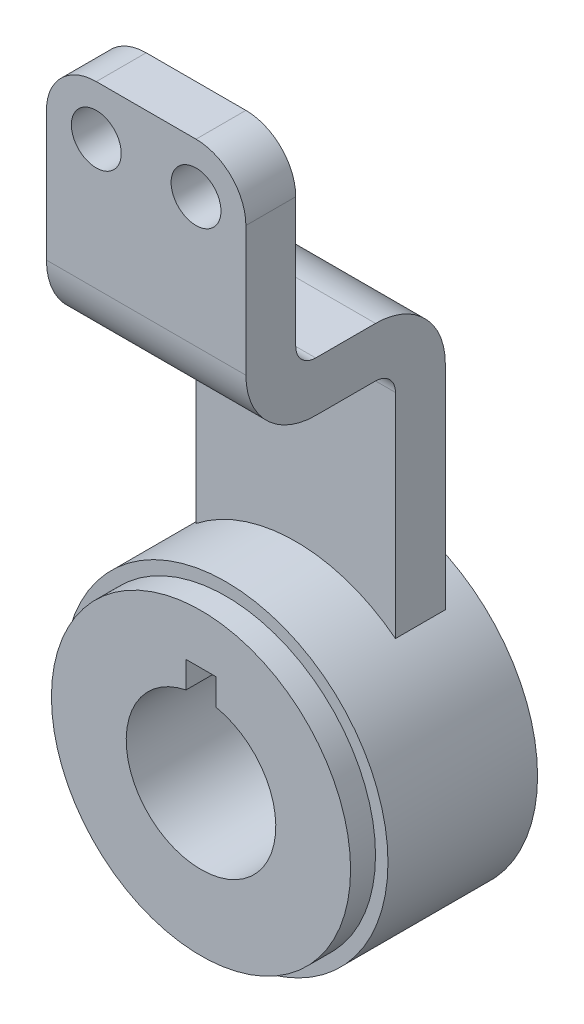
ISO-10303-21;
HEADER;
FILE_DESCRIPTION(('STEP AP214'),'2;1');
FILE_NAME('part.step','',(''),(''),'','','');
FILE_SCHEMA(('AUTOMOTIVE_DESIGN { 1 0 10303 214 1 1 1 1 }'));
ENDSEC;
DATA;
#1=APPLICATION_CONTEXT('core data for automotive mechanical design processes');
#2=APPLICATION_PROTOCOL_DEFINITION('international standard','automotive_design',2000,#1);
#3=PRODUCT_CONTEXT('',#1,'mechanical');
#4=PRODUCT('Part','Part','',(#3));
#5=PRODUCT_RELATED_PRODUCT_CATEGORY('part','',(#4));
#6=PRODUCT_DEFINITION_FORMATION('','',#4);
#7=PRODUCT_DEFINITION_CONTEXT('part definition',#1,'design');
#8=PRODUCT_DEFINITION('design','',#6,#7);
#9=PRODUCT_DEFINITION_SHAPE('','',#8);
#10=(LENGTH_UNIT() NAMED_UNIT(*) SI_UNIT(.MILLI.,.METRE.));
#11=(NAMED_UNIT(*) PLANE_ANGLE_UNIT() SI_UNIT($,.RADIAN.));
#12=(NAMED_UNIT(*) SI_UNIT($,.STERADIAN.) SOLID_ANGLE_UNIT());
#13=UNCERTAINTY_MEASURE_WITH_UNIT(LENGTH_MEASURE(1.E-05),#10,'distance_accuracy_value','');
#14=(GEOMETRIC_REPRESENTATION_CONTEXT(3) GLOBAL_UNCERTAINTY_ASSIGNED_CONTEXT((#13)) GLOBAL_UNIT_ASSIGNED_CONTEXT((#10,
#11,#12)) REPRESENTATION_CONTEXT('',''));
#15=CARTESIAN_POINT('',(0.,0.,0.));
#16=DIRECTION('',(0.,0.,1.));
#17=DIRECTION('',(1.,0.,0.));
#18=AXIS2_PLACEMENT_3D('',#15,#16,#17);
#19=CARTESIAN_POINT('',(0.,0.,16.));
#20=DIRECTION('',(0.,0.,1.));
#21=DIRECTION('',(1.,0.,0.));
#22=AXIS2_PLACEMENT_3D('',#19,#20,#21);
#23=PLANE('',#22);
#24=DIRECTION('',(0.,1.,0.));
#25=VECTOR('',#24,1.);
#26=CARTESIAN_POINT('',(20.,82.3606797749979,16.));
#27=LINE('',#26,#25);
#28=CARTESIAN_POINT('',(20.,25.617376914899,16.));
#29=VERTEX_POINT('',#28);
#30=CARTESIAN_POINT('',(20.,68.3606797749979,16.));
#31=VERTEX_POINT('',#30);
#32=EDGE_CURVE('E172',#29,#31,#27,.T.);
#33=ORIENTED_EDGE('',*,*,#32,.T.);
#34=DIRECTION('',(-1.,0.,0.));
#35=VECTOR('',#34,1.);
#36=CARTESIAN_POINT('',(0.,68.3606797749979,16.));
#37=LINE('',#36,#35);
#38=CARTESIAN_POINT('',(-20.,68.3606797749979,16.));
#39=VERTEX_POINT('',#38);
#40=EDGE_CURVE('E241',#31,#39,#37,.T.);
#41=ORIENTED_EDGE('',*,*,#40,.T.);
#42=DIRECTION('',(0.,-1.,0.));
#43=VECTOR('',#42,1.);
#44=CARTESIAN_POINT('',(-20.,22.3606797749979,16.));
#45=LINE('',#44,#43);
#46=CARTESIAN_POINT('',(-20.,25.617376914899,16.));
#47=VERTEX_POINT('',#46);
#48=EDGE_CURVE('E286',#39,#47,#45,.T.);
#49=ORIENTED_EDGE('',*,*,#48,.T.);
#50=CARTESIAN_POINT('',(0.,0.,16.));
#51=DIRECTION('',(0.,0.,1.));
#52=DIRECTION('',(1.,0.,0.));
#53=AXIS2_PLACEMENT_3D('',#50,#51,#52);
#54=CIRCLE('',#53,32.5);
#55=EDGE_CURVE('E183',#29,#47,#54,.T.);
#56=ORIENTED_EDGE('',*,*,#55,.F.);
#57=EDGE_LOOP('',(#33,#41,#49,#56));
#58=FACE_BOUND('',#57,.T.);
#59=ADVANCED_FACE('F39',(#58),#23,.T.);
#60=CARTESIAN_POINT('',(0.,0.,30.));
#61=DIRECTION('',(0.,0.,1.));
#62=DIRECTION('',(1.,0.,0.));
#63=AXIS2_PLACEMENT_3D('',#60,#61,#62);
#64=PLANE('',#63);
#65=CARTESIAN_POINT('',(0.,0.,30.));
#66=DIRECTION('',(0.,0.,1.));
#67=DIRECTION('',(1.,0.,0.));
#68=AXIS2_PLACEMENT_3D('',#65,#66,#67);
#69=CIRCLE('',#68,30.);
#70=CARTESIAN_POINT('',(30.,0.,30.));
#71=VERTEX_POINT('',#70);
#72=EDGE_CURVE('E188',#71,#71,#69,.T.);
#73=ORIENTED_EDGE('',*,*,#72,.F.);
#74=EDGE_LOOP('',(#73));
#75=FACE_BOUND('',#74,.T.);
#76=CARTESIAN_POINT('',(0.,0.,30.));
#77=DIRECTION('',(0.,0.,1.));
#78=DIRECTION('',(1.,0.,0.));
#79=AXIS2_PLACEMENT_3D('',#76,#77,#78);
#80=CIRCLE('',#79,32.5);
#81=CARTESIAN_POINT('',(32.5,0.,30.));
#82=VERTEX_POINT('',#81);
#83=EDGE_CURVE('E194',#82,#82,#80,.T.);
#84=ORIENTED_EDGE('',*,*,#83,.T.);
#85=EDGE_LOOP('',(#84));
#86=FACE_BOUND('',#85,.T.);
#87=ADVANCED_FACE('F345',(#75,#86),#64,.T.);
#88=CARTESIAN_POINT('',(0.,0.,0.));
#89=DIRECTION('',(0.,0.,1.));
#90=DIRECTION('',(1.,0.,0.));
#91=AXIS2_PLACEMENT_3D('',#88,#89,#90);
#92=PLANE('',#91);
#93=CARTESIAN_POINT('',(0.,0.,0.));
#94=DIRECTION('',(0.,0.,1.));
#95=DIRECTION('',(1.,0.,0.));
#96=AXIS2_PLACEMENT_3D('',#93,#94,#95);
#97=CIRCLE('',#96,32.5);
#98=CARTESIAN_POINT('',(32.5,0.,0.));
#99=VERTEX_POINT('',#98);
#100=EDGE_CURVE('E199',#99,#99,#97,.T.);
#101=ORIENTED_EDGE('',*,*,#100,.F.);
#102=EDGE_LOOP('',(#101));
#103=FACE_BOUND('',#102,.T.);
#104=DIRECTION('',(0.,1.,0.));
#105=VECTOR('',#104,1.);
#106=CARTESIAN_POINT('',(3.,14.6969384566991,0.));
#107=LINE('',#106,#105);
#108=CARTESIAN_POINT('',(3.,14.6969384566991,0.));
#109=VERTEX_POINT('',#108);
#110=CARTESIAN_POINT('',(3.,20.,0.));
#111=VERTEX_POINT('',#110);
#112=EDGE_CURVE('E309',#109,#111,#107,.T.);
#113=ORIENTED_EDGE('',*,*,#112,.T.);
#114=DIRECTION('',(-1.,0.,0.));
#115=VECTOR('',#114,1.);
#116=CARTESIAN_POINT('',(-3.,20.,0.));
#117=LINE('',#116,#115);
#118=CARTESIAN_POINT('',(-3.,20.,0.));
#119=VERTEX_POINT('',#118);
#120=EDGE_CURVE('E313',#111,#119,#117,.T.);
#121=ORIENTED_EDGE('',*,*,#120,.T.);
#122=DIRECTION('',(0.,-1.,0.));
#123=VECTOR('',#122,1.);
#124=CARTESIAN_POINT('',(-3.,14.6969384566991,0.));
#125=LINE('',#124,#123);
#126=CARTESIAN_POINT('',(-3.,14.6969384566991,0.));
#127=VERTEX_POINT('',#126);
#128=EDGE_CURVE('E320',#119,#127,#125,.T.);
#129=ORIENTED_EDGE('',*,*,#128,.T.);
#130=CARTESIAN_POINT('',(0.,0.,0.));
#131=DIRECTION('',(0.,0.,1.));
#132=DIRECTION('',(1.,0.,0.));
#133=AXIS2_PLACEMENT_3D('',#130,#131,#132);
#134=CIRCLE('',#133,15.);
#135=EDGE_CURVE('E318',#127,#109,#134,.T.);
#136=ORIENTED_EDGE('',*,*,#135,.T.);
#137=EDGE_LOOP('',(#113,#121,#129,#136));
#138=FACE_BOUND('',#137,.T.);
#139=ADVANCED_FACE('F339',(#103,#138),#92,.F.);
#140=CARTESIAN_POINT('',(0.,0.,30.));
#141=DIRECTION('',(0.,0.,-1.));
#142=DIRECTION('',(-1.,0.,0.));
#143=AXIS2_PLACEMENT_3D('',#140,#141,#142);
#144=CYLINDRICAL_SURFACE('',#143,32.5);
#145=DIRECTION('',(0.,0.,-1.));
#146=VECTOR('',#145,1.);
#147=CARTESIAN_POINT('',(20.,25.617376914899,30.));
#148=LINE('',#147,#146);
#149=CARTESIAN_POINT('',(20.,25.617376914899,6.));
#150=VERTEX_POINT('',#149);
#151=EDGE_CURVE('E184',#29,#150,#148,.T.);
#152=ORIENTED_EDGE('',*,*,#151,.F.);
#153=ORIENTED_EDGE('',*,*,#55,.T.);
#154=DIRECTION('',(0.,0.,-1.));
#155=VECTOR('',#154,1.);
#156=CARTESIAN_POINT('',(-20.,25.617376914899,30.));
#157=LINE('',#156,#155);
#158=CARTESIAN_POINT('',(-20.,25.617376914899,6.));
#159=VERTEX_POINT('',#158);
#160=EDGE_CURVE('E166',#159,#47,#157,.F.);
#161=ORIENTED_EDGE('',*,*,#160,.F.);
#162=CARTESIAN_POINT('',(0.,0.,6.));
#163=DIRECTION('',(0.,0.,1.));
#164=DIRECTION('',(1.,0.,0.));
#165=AXIS2_PLACEMENT_3D('',#162,#163,#164);
#166=CIRCLE('',#165,32.5);
#167=EDGE_CURVE('E181',#150,#159,#166,.T.);
#168=ORIENTED_EDGE('',*,*,#167,.F.);
#169=EDGE_LOOP('',(#152,#153,#161,#168));
#170=FACE_BOUND('',#169,.T.);
#171=ORIENTED_EDGE('',*,*,#83,.F.);
#172=EDGE_LOOP('',(#171));
#173=FACE_BOUND('',#172,.T.);
#174=ORIENTED_EDGE('',*,*,#100,.T.);
#175=EDGE_LOOP('',(#174));
#176=FACE_BOUND('',#175,.T.);
#177=ADVANCED_FACE('F177',(#170,#173,#176),#144,.T.);
#178=CARTESIAN_POINT('',(3.,14.6969384566991,30.));
#179=DIRECTION('',(-1.,0.,0.));
#180=DIRECTION('',(0.,0.,1.));
#181=AXIS2_PLACEMENT_3D('',#178,#179,#180);
#182=PLANE('',#181);
#183=ORIENTED_EDGE('',*,*,#112,.F.);
#184=DIRECTION('',(0.,0.,-1.));
#185=VECTOR('',#184,1.);
#186=CARTESIAN_POINT('',(3.,14.6969384566991,30.));
#187=LINE('',#186,#185);
#188=CARTESIAN_POINT('',(3.,14.6969384566991,35.));
#189=VERTEX_POINT('',#188);
#190=EDGE_CURVE('E324',#189,#109,#187,.T.);
#191=ORIENTED_EDGE('',*,*,#190,.F.);
#192=DIRECTION('',(0.,1.,0.));
#193=VECTOR('',#192,1.);
#194=CARTESIAN_POINT('',(3.,20.,35.));
#195=LINE('',#194,#193);
#196=CARTESIAN_POINT('',(3.,20.,35.));
#197=VERTEX_POINT('',#196);
#198=EDGE_CURVE('E299',#189,#197,#195,.T.);
#199=ORIENTED_EDGE('',*,*,#198,.T.);
#200=DIRECTION('',(0.,0.,-1.));
#201=VECTOR('',#200,1.);
#202=CARTESIAN_POINT('',(3.,20.,30.));
#203=LINE('',#202,#201);
#204=EDGE_CURVE('E327',#197,#111,#203,.T.);
#205=ORIENTED_EDGE('',*,*,#204,.T.);
#206=EDGE_LOOP('',(#183,#191,#199,#205));
#207=FACE_BOUND('',#206,.T.);
#208=ADVANCED_FACE('F349',(#207),#182,.T.);
#209=CARTESIAN_POINT('',(-3.,20.,30.));
#210=DIRECTION('',(0.,-1.,0.));
#211=DIRECTION('',(0.,0.,-1.));
#212=AXIS2_PLACEMENT_3D('',#209,#210,#211);
#213=PLANE('',#212);
#214=ORIENTED_EDGE('',*,*,#120,.F.);
#215=ORIENTED_EDGE('',*,*,#204,.F.);
#216=DIRECTION('',(-1.,0.,0.));
#217=VECTOR('',#216,1.);
#218=CARTESIAN_POINT('',(-3.,20.,35.));
#219=LINE('',#218,#217);
#220=CARTESIAN_POINT('',(-3.,20.,35.));
#221=VERTEX_POINT('',#220);
#222=EDGE_CURVE('E305',#197,#221,#219,.T.);
#223=ORIENTED_EDGE('',*,*,#222,.T.);
#224=DIRECTION('',(0.,0.,-1.));
#225=VECTOR('',#224,1.);
#226=CARTESIAN_POINT('',(-3.,20.,30.));
#227=LINE('',#226,#225);
#228=EDGE_CURVE('E330',#221,#119,#227,.T.);
#229=ORIENTED_EDGE('',*,*,#228,.T.);
#230=EDGE_LOOP('',(#214,#215,#223,#229));
#231=FACE_BOUND('',#230,.T.);
#232=ADVANCED_FACE('F358',(#231),#213,.T.);
#233=CARTESIAN_POINT('',(-3.,14.6969384566991,30.));
#234=DIRECTION('',(1.,0.,0.));
#235=DIRECTION('',(0.,0.,-1.));
#236=AXIS2_PLACEMENT_3D('',#233,#234,#235);
#237=PLANE('',#236);
#238=ORIENTED_EDGE('',*,*,#128,.F.);
#239=ORIENTED_EDGE('',*,*,#228,.F.);
#240=DIRECTION('',(0.,-1.,0.));
#241=VECTOR('',#240,1.);
#242=CARTESIAN_POINT('',(-3.,14.6969384566991,35.));
#243=LINE('',#242,#241);
#244=CARTESIAN_POINT('',(-3.,14.6969384566991,35.));
#245=VERTEX_POINT('',#244);
#246=EDGE_CURVE('E304',#221,#245,#243,.T.);
#247=ORIENTED_EDGE('',*,*,#246,.T.);
#248=DIRECTION('',(0.,0.,-1.));
#249=VECTOR('',#248,1.);
#250=CARTESIAN_POINT('',(-3.,14.6969384566991,30.));
#251=LINE('',#250,#249);
#252=EDGE_CURVE('E329',#245,#127,#251,.T.);
#253=ORIENTED_EDGE('',*,*,#252,.T.);
#254=EDGE_LOOP('',(#238,#239,#247,#253));
#255=FACE_BOUND('',#254,.T.);
#256=ADVANCED_FACE('F360',(#255),#237,.T.);
#257=CARTESIAN_POINT('',(0.,0.,30.));
#258=DIRECTION('',(0.,0.,-1.));
#259=DIRECTION('',(-1.,0.,0.));
#260=AXIS2_PLACEMENT_3D('',#257,#258,#259);
#261=CYLINDRICAL_SURFACE('',#260,15.);
#262=ORIENTED_EDGE('',*,*,#135,.F.);
#263=ORIENTED_EDGE('',*,*,#252,.F.);
#264=CARTESIAN_POINT('',(0.,0.,35.));
#265=DIRECTION('',(0.,0.,1.));
#266=DIRECTION('',(1.,0.,0.));
#267=AXIS2_PLACEMENT_3D('',#264,#265,#266);
#268=CIRCLE('',#267,15.);
#269=EDGE_CURVE('E298',#245,#189,#268,.T.);
#270=ORIENTED_EDGE('',*,*,#269,.T.);
#271=ORIENTED_EDGE('',*,*,#190,.T.);
#272=EDGE_LOOP('',(#262,#263,#270,#271));
#273=FACE_BOUND('',#272,.T.);
#274=ADVANCED_FACE('F350',(#273),#261,.F.);
#275=CARTESIAN_POINT('',(0.,0.,35.));
#276=DIRECTION('',(0.,0.,1.));
#277=DIRECTION('',(1.,0.,0.));
#278=AXIS2_PLACEMENT_3D('',#275,#276,#277);
#279=PLANE('',#278);
#280=CARTESIAN_POINT('',(0.,0.,35.));
#281=DIRECTION('',(0.,0.,1.));
#282=DIRECTION('',(1.,0.,0.));
#283=AXIS2_PLACEMENT_3D('',#280,#281,#282);
#284=CIRCLE('',#283,30.);
#285=CARTESIAN_POINT('',(30.,0.,35.));
#286=VERTEX_POINT('',#285);
#287=EDGE_CURVE('E308',#286,#286,#284,.T.);
#288=ORIENTED_EDGE('',*,*,#287,.T.);
#289=EDGE_LOOP('',(#288));
#290=FACE_BOUND('',#289,.T.);
#291=ORIENTED_EDGE('',*,*,#198,.F.);
#292=ORIENTED_EDGE('',*,*,#269,.F.);
#293=ORIENTED_EDGE('',*,*,#246,.F.);
#294=ORIENTED_EDGE('',*,*,#222,.F.);
#295=EDGE_LOOP('',(#291,#292,#293,#294));
#296=FACE_BOUND('',#295,.T.);
#297=ADVANCED_FACE('F351',(#290,#296),#279,.T.);
#298=CARTESIAN_POINT('',(0.,0.,35.));
#299=DIRECTION('',(0.,0.,-1.));
#300=DIRECTION('',(-1.,0.,0.));
#301=AXIS2_PLACEMENT_3D('',#298,#299,#300);
#302=CYLINDRICAL_SURFACE('',#301,30.);
#303=ORIENTED_EDGE('',*,*,#287,.F.);
#304=EDGE_LOOP('',(#303));
#305=FACE_BOUND('',#304,.T.);
#306=ORIENTED_EDGE('',*,*,#72,.T.);
#307=EDGE_LOOP('',(#306));
#308=FACE_BOUND('',#307,.T.);
#309=ADVANCED_FACE('F395',(#305,#308),#302,.T.);
#310=CARTESIAN_POINT('',(20.,82.3606797749979,16.));
#311=DIRECTION('',(-1.,0.,0.));
#312=DIRECTION('',(0.,-1.,0.));
#313=AXIS2_PLACEMENT_3D('',#310,#311,#312);
#314=PLANE('',#313);
#315=DIRECTION('',(0.,1.,0.));
#316=VECTOR('',#315,1.);
#317=CARTESIAN_POINT('',(20.,72.3606797749979,46.));
#318=LINE('',#317,#316);
#319=CARTESIAN_POINT('',(20.,86.3606797749979,46.));
#320=VERTEX_POINT('',#319);
#321=CARTESIAN_POINT('',(20.,112.360679774998,46.));
#322=VERTEX_POINT('',#321);
#323=EDGE_CURVE('E283',#320,#322,#318,.T.);
#324=ORIENTED_EDGE('',*,*,#323,.F.);
#325=CARTESIAN_POINT('',(20.,86.3606797749979,32.));
#326=DIRECTION('',(-1.,0.,0.));
#327=DIRECTION('',(0.,-1.,0.));
#328=AXIS2_PLACEMENT_3D('',#325,#326,#327);
#329=CIRCLE('',#328,14.);
#330=CARTESIAN_POINT('',(20.,72.3606797749979,32.));
#331=VERTEX_POINT('',#330);
#332=EDGE_CURVE('E234',#320,#331,#329,.F.);
#333=ORIENTED_EDGE('',*,*,#332,.T.);
#334=DIRECTION('',(0.,0.,-1.));
#335=VECTOR('',#334,1.);
#336=CARTESIAN_POINT('',(20.,72.3606797749979,6.));
#337=LINE('',#336,#335);
#338=CARTESIAN_POINT('',(20.,72.3606797749979,20.));
#339=VERTEX_POINT('',#338);
#340=EDGE_CURVE('E278',#331,#339,#337,.T.);
#341=ORIENTED_EDGE('',*,*,#340,.T.);
#342=CARTESIAN_POINT('',(20.,68.3606797749979,20.));
#343=DIRECTION('',(-1.,0.,0.));
#344=DIRECTION('',(0.,-1.,0.));
#345=AXIS2_PLACEMENT_3D('',#342,#343,#344);
#346=CIRCLE('',#345,4.);
#347=EDGE_CURVE('E247',#339,#31,#346,.T.);
#348=ORIENTED_EDGE('',*,*,#347,.T.);
#349=ORIENTED_EDGE('',*,*,#32,.F.);
#350=ORIENTED_EDGE('',*,*,#151,.T.);
#351=DIRECTION('',(0.,1.,0.));
#352=VECTOR('',#351,1.);
#353=CARTESIAN_POINT('',(20.,82.3606797749979,6.));
#354=LINE('',#353,#352);
#355=CARTESIAN_POINT('',(20.,68.3606797749979,6.));
#356=VERTEX_POINT('',#355);
#357=EDGE_CURVE('E174',#150,#356,#354,.T.);
#358=ORIENTED_EDGE('',*,*,#357,.T.);
#359=CARTESIAN_POINT('',(20.,68.3606797749979,20.));
#360=DIRECTION('',(-1.,0.,0.));
#361=DIRECTION('',(0.,-1.,0.));
#362=AXIS2_PLACEMENT_3D('',#359,#360,#361);
#363=CIRCLE('',#362,14.);
#364=CARTESIAN_POINT('',(20.,82.3606797749979,20.));
#365=VERTEX_POINT('',#364);
#366=EDGE_CURVE('E226',#356,#365,#363,.F.);
#367=ORIENTED_EDGE('',*,*,#366,.T.);
#368=DIRECTION('',(0.,0.,-1.));
#369=VECTOR('',#368,1.);
#370=CARTESIAN_POINT('',(20.,82.3606797749979,16.));
#371=LINE('',#370,#369);
#372=CARTESIAN_POINT('',(20.,82.3606797749979,32.));
#373=VERTEX_POINT('',#372);
#374=EDGE_CURVE('E295',#373,#365,#371,.T.);
#375=ORIENTED_EDGE('',*,*,#374,.F.);
#376=CARTESIAN_POINT('',(20.,86.3606797749979,32.));
#377=DIRECTION('',(-1.,0.,0.));
#378=DIRECTION('',(0.,-1.,0.));
#379=AXIS2_PLACEMENT_3D('',#376,#377,#378);
#380=CIRCLE('',#379,4.);
#381=CARTESIAN_POINT('',(20.,86.3606797749979,36.));
#382=VERTEX_POINT('',#381);
#383=EDGE_CURVE('E48',#373,#382,#380,.T.);
#384=ORIENTED_EDGE('',*,*,#383,.T.);
#385=DIRECTION('',(0.,1.,0.));
#386=VECTOR('',#385,1.);
#387=CARTESIAN_POINT('',(20.,72.3606797749979,36.));
#388=LINE('',#387,#386);
#389=CARTESIAN_POINT('',(20.,112.360679774998,36.));
#390=VERTEX_POINT('',#389);
#391=EDGE_CURVE('E258',#382,#390,#388,.T.);
#392=ORIENTED_EDGE('',*,*,#391,.T.);
#393=DIRECTION('',(0.,0.,1.));
#394=VECTOR('',#393,1.);
#395=CARTESIAN_POINT('',(20.,112.360679774998,46.));
#396=LINE('',#395,#394);
#397=EDGE_CURVE('E202',#390,#322,#396,.T.);
#398=ORIENTED_EDGE('',*,*,#397,.T.);
#399=EDGE_LOOP('',(#324,#333,#341,#348,#349,#350,#358,#367,#375,#384,#392,#398));
#400=FACE_BOUND('',#399,.T.);
#401=ADVANCED_FACE('F390',(#400),#314,.F.);
#402=CARTESIAN_POINT('',(-20.,22.3606797749979,16.));
#403=DIRECTION('',(1.,0.,0.));
#404=DIRECTION('',(0.,0.,-1.));
#405=AXIS2_PLACEMENT_3D('',#402,#403,#404);
#406=PLANE('',#405);
#407=ORIENTED_EDGE('',*,*,#48,.F.);
#408=CARTESIAN_POINT('',(-20.,68.3606797749979,20.));
#409=DIRECTION('',(1.,0.,0.));
#410=DIRECTION('',(0.,0.,-1.));
#411=AXIS2_PLACEMENT_3D('',#408,#409,#410);
#412=CIRCLE('',#411,4.);
#413=CARTESIAN_POINT('',(-20.,72.3606797749979,20.));
#414=VERTEX_POINT('',#413);
#415=EDGE_CURVE('E246',#39,#414,#412,.T.);
#416=ORIENTED_EDGE('',*,*,#415,.T.);
#417=DIRECTION('',(0.,0.,1.));
#418=VECTOR('',#417,1.);
#419=CARTESIAN_POINT('',(-20.,72.3606797749979,6.));
#420=LINE('',#419,#418);
#421=CARTESIAN_POINT('',(-20.,72.3606797749979,32.));
#422=VERTEX_POINT('',#421);
#423=EDGE_CURVE('E277',#414,#422,#420,.T.);
#424=ORIENTED_EDGE('',*,*,#423,.T.);
#425=CARTESIAN_POINT('',(-20.,86.3606797749979,32.));
#426=DIRECTION('',(1.,0.,0.));
#427=DIRECTION('',(0.,0.,-1.));
#428=AXIS2_PLACEMENT_3D('',#425,#426,#427);
#429=CIRCLE('',#428,14.);
#430=CARTESIAN_POINT('',(-20.,86.3606797749979,46.));
#431=VERTEX_POINT('',#430);
#432=EDGE_CURVE('E237',#422,#431,#429,.F.);
#433=ORIENTED_EDGE('',*,*,#432,.T.);
#434=DIRECTION('',(0.,1.,0.));
#435=VECTOR('',#434,1.);
#436=CARTESIAN_POINT('',(-20.,72.3606797749979,46.));
#437=LINE('',#436,#435);
#438=CARTESIAN_POINT('',(-20.,112.360679774998,46.));
#439=VERTEX_POINT('',#438);
#440=EDGE_CURVE('E285',#431,#439,#437,.T.);
#441=ORIENTED_EDGE('',*,*,#440,.T.);
#442=DIRECTION('',(0.,0.,1.));
#443=VECTOR('',#442,1.);
#444=CARTESIAN_POINT('',(-20.,112.360679774998,36.));
#445=LINE('',#444,#443);
#446=CARTESIAN_POINT('',(-20.,112.360679774998,36.));
#447=VERTEX_POINT('',#446);
#448=EDGE_CURVE('E218',#439,#447,#445,.F.);
#449=ORIENTED_EDGE('',*,*,#448,.T.);
#450=DIRECTION('',(0.,1.,0.));
#451=VECTOR('',#450,1.);
#452=CARTESIAN_POINT('',(-20.,72.3606797749979,36.));
#453=LINE('',#452,#451);
#454=CARTESIAN_POINT('',(-20.,86.3606797749979,36.));
#455=VERTEX_POINT('',#454);
#456=EDGE_CURVE('E266',#455,#447,#453,.T.);
#457=ORIENTED_EDGE('',*,*,#456,.F.);
#458=CARTESIAN_POINT('',(-20.,86.3606797749979,32.));
#459=DIRECTION('',(1.,0.,0.));
#460=DIRECTION('',(0.,0.,-1.));
#461=AXIS2_PLACEMENT_3D('',#458,#459,#460);
#462=CIRCLE('',#461,4.);
#463=CARTESIAN_POINT('',(-20.,82.3606797749979,32.));
#464=VERTEX_POINT('',#463);
#465=EDGE_CURVE('E11',#455,#464,#462,.T.);
#466=ORIENTED_EDGE('',*,*,#465,.T.);
#467=DIRECTION('',(0.,0.,-1.));
#468=VECTOR('',#467,1.);
#469=CARTESIAN_POINT('',(-20.,82.3606797749979,16.));
#470=LINE('',#469,#468);
#471=CARTESIAN_POINT('',(-20.,82.3606797749979,20.));
#472=VERTEX_POINT('',#471);
#473=EDGE_CURVE('E293',#464,#472,#470,.T.);
#474=ORIENTED_EDGE('',*,*,#473,.T.);
#475=CARTESIAN_POINT('',(-20.,68.3606797749979,20.));
#476=DIRECTION('',(1.,0.,0.));
#477=DIRECTION('',(0.,0.,-1.));
#478=AXIS2_PLACEMENT_3D('',#475,#476,#477);
#479=CIRCLE('',#478,14.);
#480=CARTESIAN_POINT('',(-20.,68.3606797749979,6.));
#481=VERTEX_POINT('',#480);
#482=EDGE_CURVE('E167',#472,#481,#479,.F.);
#483=ORIENTED_EDGE('',*,*,#482,.T.);
#484=DIRECTION('',(0.,-1.,0.));
#485=VECTOR('',#484,1.);
#486=CARTESIAN_POINT('',(-20.,22.3606797749979,6.));
#487=LINE('',#486,#485);
#488=EDGE_CURVE('E165',#481,#159,#487,.T.);
#489=ORIENTED_EDGE('',*,*,#488,.T.);
#490=ORIENTED_EDGE('',*,*,#160,.T.);
#491=EDGE_LOOP('',(#407,#416,#424,#433,#441,#449,#457,#466,#474,#483,#489,#490));
#492=FACE_BOUND('',#491,.T.);
#493=ADVANCED_FACE('F170',(#492),#406,.F.);
#494=CARTESIAN_POINT('',(-20.,82.3606797749979,16.));
#495=DIRECTION('',(0.,-1.,0.));
#496=DIRECTION('',(0.,0.,-1.));
#497=AXIS2_PLACEMENT_3D('',#494,#495,#496);
#498=PLANE('',#497);
#499=ORIENTED_EDGE('',*,*,#473,.F.);
#500=DIRECTION('',(1.,0.,0.));
#501=VECTOR('',#500,1.);
#502=CARTESIAN_POINT('',(-20.,82.3606797749979,32.));
#503=LINE('',#502,#501);
#504=EDGE_CURVE('E249',#464,#373,#503,.T.);
#505=ORIENTED_EDGE('',*,*,#504,.T.);
#506=ORIENTED_EDGE('',*,*,#374,.T.);
#507=DIRECTION('',(-1.,0.,0.));
#508=VECTOR('',#507,1.);
#509=CARTESIAN_POINT('',(-20.,82.3606797749979,20.));
#510=LINE('',#509,#508);
#511=EDGE_CURVE('E224',#365,#472,#510,.T.);
#512=ORIENTED_EDGE('',*,*,#511,.T.);
#513=EDGE_LOOP('',(#499,#505,#506,#512));
#514=FACE_BOUND('',#513,.T.);
#515=ADVANCED_FACE('F381',(#514),#498,.F.);
#516=CARTESIAN_POINT('',(0.,0.,6.));
#517=DIRECTION('',(0.,0.,1.));
#518=DIRECTION('',(1.,0.,0.));
#519=AXIS2_PLACEMENT_3D('',#516,#517,#518);
#520=PLANE('',#519);
#521=ORIENTED_EDGE('',*,*,#488,.F.);
#522=DIRECTION('',(-1.,0.,0.));
#523=VECTOR('',#522,1.);
#524=CARTESIAN_POINT('',(0.,68.3606797749979,6.));
#525=LINE('',#524,#523);
#526=EDGE_CURVE('E228',#481,#356,#525,.F.);
#527=ORIENTED_EDGE('',*,*,#526,.T.);
#528=ORIENTED_EDGE('',*,*,#357,.F.);
#529=ORIENTED_EDGE('',*,*,#167,.T.);
#530=EDGE_LOOP('',(#521,#527,#528,#529));
#531=FACE_BOUND('',#530,.T.);
#532=ADVANCED_FACE('F189',(#531),#520,.F.);
#533=CARTESIAN_POINT('',(-20.,72.3606797749979,46.));
#534=DIRECTION('',(0.,0.,1.));
#535=DIRECTION('',(1.,0.,0.));
#536=AXIS2_PLACEMENT_3D('',#533,#534,#535);
#537=PLANE('',#536);
#538=CARTESIAN_POINT('',(-10.,112.360679774998,46.));
#539=DIRECTION('',(0.,0.,1.));
#540=DIRECTION('',(1.,0.,0.));
#541=AXIS2_PLACEMENT_3D('',#538,#539,#540);
#542=CIRCLE('',#541,5.);
#543=CARTESIAN_POINT('',(-5.,112.360679774998,46.));
#544=VERTEX_POINT('',#543);
#545=EDGE_CURVE('E257',#544,#544,#542,.T.);
#546=ORIENTED_EDGE('',*,*,#545,.F.);
#547=EDGE_LOOP('',(#546));
#548=FACE_BOUND('',#547,.T.);
#549=CARTESIAN_POINT('',(9.99999999999999,112.360679774998,46.));
#550=DIRECTION('',(0.,0.,1.));
#551=DIRECTION('',(1.,0.,0.));
#552=AXIS2_PLACEMENT_3D('',#549,#550,#551);
#553=CIRCLE('',#552,5.00000000000001);
#554=CARTESIAN_POINT('',(15.,112.360679774998,46.));
#555=VERTEX_POINT('',#554);
#556=EDGE_CURVE('E261',#555,#555,#553,.T.);
#557=ORIENTED_EDGE('',*,*,#556,.F.);
#558=EDGE_LOOP('',(#557));
#559=FACE_BOUND('',#558,.T.);
#560=ORIENTED_EDGE('',*,*,#440,.F.);
#561=DIRECTION('',(1.,0.,0.));
#562=VECTOR('',#561,1.);
#563=CARTESIAN_POINT('',(20.,86.3606797749979,46.));
#564=LINE('',#563,#562);
#565=EDGE_CURVE('E233',#431,#320,#564,.T.);
#566=ORIENTED_EDGE('',*,*,#565,.T.);
#567=ORIENTED_EDGE('',*,*,#323,.T.);
#568=CARTESIAN_POINT('',(9.99999999999999,112.360679774998,46.));
#569=DIRECTION('',(0.,0.,1.));
#570=DIRECTION('',(1.,0.,0.));
#571=AXIS2_PLACEMENT_3D('',#568,#569,#570);
#572=CIRCLE('',#571,10.);
#573=CARTESIAN_POINT('',(9.99999999999999,122.360679774998,46.));
#574=VERTEX_POINT('',#573);
#575=EDGE_CURVE('E210',#322,#574,#572,.T.);
#576=ORIENTED_EDGE('',*,*,#575,.T.);
#577=DIRECTION('',(1.,0.,0.));
#578=VECTOR('',#577,1.);
#579=CARTESIAN_POINT('',(-20.,122.360679774998,46.));
#580=LINE('',#579,#578);
#581=CARTESIAN_POINT('',(-10.,122.360679774998,46.));
#582=VERTEX_POINT('',#581);
#583=EDGE_CURVE('E271',#582,#574,#580,.T.);
#584=ORIENTED_EDGE('',*,*,#583,.F.);
#585=CARTESIAN_POINT('',(-10.,112.360679774998,46.));
#586=DIRECTION('',(0.,0.,1.));
#587=DIRECTION('',(1.,0.,0.));
#588=AXIS2_PLACEMENT_3D('',#585,#586,#587);
#589=CIRCLE('',#588,10.);
#590=EDGE_CURVE('E201',#582,#439,#589,.T.);
#591=ORIENTED_EDGE('',*,*,#590,.T.);
#592=EDGE_LOOP('',(#560,#566,#567,#576,#584,#591));
#593=FACE_BOUND('',#592,.T.);
#594=ADVANCED_FACE('F379',(#548,#559,#593),#537,.T.);
#595=CARTESIAN_POINT('',(0.,72.3606797749979,0.));
#596=DIRECTION('',(0.,1.,0.));
#597=DIRECTION('',(0.,0.,1.));
#598=AXIS2_PLACEMENT_3D('',#595,#596,#597);
#599=PLANE('',#598);
#600=ORIENTED_EDGE('',*,*,#423,.F.);
#601=DIRECTION('',(-1.,0.,0.));
#602=VECTOR('',#601,1.);
#603=CARTESIAN_POINT('',(0.,72.3606797749979,20.));
#604=LINE('',#603,#602);
#605=EDGE_CURVE('E242',#414,#339,#604,.F.);
#606=ORIENTED_EDGE('',*,*,#605,.T.);
#607=ORIENTED_EDGE('',*,*,#340,.F.);
#608=DIRECTION('',(1.,0.,0.));
#609=VECTOR('',#608,1.);
#610=CARTESIAN_POINT('',(-20.,72.3606797749979,32.));
#611=LINE('',#610,#609);
#612=EDGE_CURVE('E236',#331,#422,#611,.F.);
#613=ORIENTED_EDGE('',*,*,#612,.T.);
#614=EDGE_LOOP('',(#600,#606,#607,#613));
#615=FACE_BOUND('',#614,.T.);
#616=ADVANCED_FACE('F515',(#615),#599,.F.);
#617=CARTESIAN_POINT('',(-20.,72.3606797749979,36.));
#618=DIRECTION('',(0.,0.,-1.));
#619=DIRECTION('',(-1.,0.,0.));
#620=AXIS2_PLACEMENT_3D('',#617,#618,#619);
#621=PLANE('',#620);
#622=CARTESIAN_POINT('',(-10.,112.360679774998,36.));
#623=DIRECTION('',(0.,0.,-1.));
#624=DIRECTION('',(-1.,0.,0.));
#625=AXIS2_PLACEMENT_3D('',#622,#623,#624);
#626=CIRCLE('',#625,5.);
#627=CARTESIAN_POINT('',(-15.,112.360679774998,36.));
#628=VERTEX_POINT('',#627);
#629=EDGE_CURVE('E43',#628,#628,#626,.T.);
#630=ORIENTED_EDGE('',*,*,#629,.F.);
#631=EDGE_LOOP('',(#630));
#632=FACE_BOUND('',#631,.T.);
#633=CARTESIAN_POINT('',(9.99999999999999,112.360679774998,36.));
#634=DIRECTION('',(0.,0.,-1.));
#635=DIRECTION('',(-1.,0.,0.));
#636=AXIS2_PLACEMENT_3D('',#633,#634,#635);
#637=CIRCLE('',#636,5.00000000000001);
#638=CARTESIAN_POINT('',(4.99999999999998,112.360679774998,36.));
#639=VERTEX_POINT('',#638);
#640=EDGE_CURVE('E251',#639,#639,#637,.T.);
#641=ORIENTED_EDGE('',*,*,#640,.F.);
#642=EDGE_LOOP('',(#641));
#643=FACE_BOUND('',#642,.T.);
#644=ORIENTED_EDGE('',*,*,#391,.F.);
#645=DIRECTION('',(1.,0.,0.));
#646=VECTOR('',#645,1.);
#647=CARTESIAN_POINT('',(-20.,86.3606797749979,36.));
#648=LINE('',#647,#646);
#649=EDGE_CURVE('E57',#382,#455,#648,.F.);
#650=ORIENTED_EDGE('',*,*,#649,.T.);
#651=ORIENTED_EDGE('',*,*,#456,.T.);
#652=CARTESIAN_POINT('',(-10.,112.360679774998,36.));
#653=DIRECTION('',(0.,0.,-1.));
#654=DIRECTION('',(-1.,0.,0.));
#655=AXIS2_PLACEMENT_3D('',#652,#653,#654);
#656=CIRCLE('',#655,10.);
#657=CARTESIAN_POINT('',(-10.,122.360679774998,36.));
#658=VERTEX_POINT('',#657);
#659=EDGE_CURVE('E211',#447,#658,#656,.T.);
#660=ORIENTED_EDGE('',*,*,#659,.T.);
#661=DIRECTION('',(1.,0.,0.));
#662=VECTOR('',#661,1.);
#663=CARTESIAN_POINT('',(-20.,122.360679774998,36.));
#664=LINE('',#663,#662);
#665=CARTESIAN_POINT('',(9.99999999999999,122.360679774998,36.));
#666=VERTEX_POINT('',#665);
#667=EDGE_CURVE('E272',#658,#666,#664,.T.);
#668=ORIENTED_EDGE('',*,*,#667,.T.);
#669=CARTESIAN_POINT('',(9.99999999999999,112.360679774998,36.));
#670=DIRECTION('',(0.,0.,-1.));
#671=DIRECTION('',(-1.,0.,0.));
#672=AXIS2_PLACEMENT_3D('',#669,#670,#671);
#673=CIRCLE('',#672,10.);
#674=EDGE_CURVE('E219',#666,#390,#673,.T.);
#675=ORIENTED_EDGE('',*,*,#674,.T.);
#676=EDGE_LOOP('',(#644,#650,#651,#660,#668,#675));
#677=FACE_BOUND('',#676,.T.);
#678=ADVANCED_FACE('F424',(#632,#643,#677),#621,.T.);
#679=CARTESIAN_POINT('',(-20.,122.360679774998,46.));
#680=DIRECTION('',(0.,1.,0.));
#681=DIRECTION('',(-1.,0.,0.));
#682=AXIS2_PLACEMENT_3D('',#679,#680,#681);
#683=PLANE('',#682);
#684=ORIENTED_EDGE('',*,*,#583,.T.);
#685=DIRECTION('',(0.,0.,1.));
#686=VECTOR('',#685,1.);
#687=CARTESIAN_POINT('',(9.99999999999999,122.360679774998,36.));
#688=LINE('',#687,#686);
#689=EDGE_CURVE('E215',#574,#666,#688,.F.);
#690=ORIENTED_EDGE('',*,*,#689,.T.);
#691=ORIENTED_EDGE('',*,*,#667,.F.);
#692=DIRECTION('',(0.,0.,1.));
#693=VECTOR('',#692,1.);
#694=CARTESIAN_POINT('',(-10.,122.360679774998,46.));
#695=LINE('',#694,#693);
#696=EDGE_CURVE('E209',#658,#582,#695,.T.);
#697=ORIENTED_EDGE('',*,*,#696,.T.);
#698=EDGE_LOOP('',(#684,#690,#691,#697));
#699=FACE_BOUND('',#698,.T.);
#700=ADVANCED_FACE('F418',(#699),#683,.T.);
#701=CARTESIAN_POINT('',(9.99999999999999,112.360679774998,16.));
#702=DIRECTION('',(0.,0.,-1.));
#703=DIRECTION('',(-1.,0.,0.));
#704=AXIS2_PLACEMENT_3D('',#701,#702,#703);
#705=CYLINDRICAL_SURFACE('',#704,10.);
#706=ORIENTED_EDGE('',*,*,#674,.F.);
#707=ORIENTED_EDGE('',*,*,#689,.F.);
#708=ORIENTED_EDGE('',*,*,#575,.F.);
#709=ORIENTED_EDGE('',*,*,#397,.F.);
#710=EDGE_LOOP('',(#706,#707,#708,#709));
#711=FACE_BOUND('',#710,.T.);
#712=ADVANCED_FACE('F425',(#711),#705,.T.);
#713=CARTESIAN_POINT('',(-10.,112.360679774998,46.));
#714=DIRECTION('',(0.,0.,-1.));
#715=DIRECTION('',(-1.,0.,0.));
#716=AXIS2_PLACEMENT_3D('',#713,#714,#715);
#717=CYLINDRICAL_SURFACE('',#716,10.);
#718=ORIENTED_EDGE('',*,*,#659,.F.);
#719=ORIENTED_EDGE('',*,*,#448,.F.);
#720=ORIENTED_EDGE('',*,*,#590,.F.);
#721=ORIENTED_EDGE('',*,*,#696,.F.);
#722=EDGE_LOOP('',(#718,#719,#720,#721));
#723=FACE_BOUND('',#722,.T.);
#724=ADVANCED_FACE('F434',(#723),#717,.T.);
#725=CARTESIAN_POINT('',(-20.,68.3606797749979,20.));
#726=DIRECTION('',(-1.,0.,0.));
#727=DIRECTION('',(0.,0.,1.));
#728=AXIS2_PLACEMENT_3D('',#725,#726,#727);
#729=CYLINDRICAL_SURFACE('',#728,14.);
#730=ORIENTED_EDGE('',*,*,#366,.F.);
#731=ORIENTED_EDGE('',*,*,#526,.F.);
#732=ORIENTED_EDGE('',*,*,#482,.F.);
#733=ORIENTED_EDGE('',*,*,#511,.F.);
#734=EDGE_LOOP('',(#730,#731,#732,#733));
#735=FACE_BOUND('',#734,.T.);
#736=ADVANCED_FACE('F442',(#735),#729,.T.);
#737=CARTESIAN_POINT('',(-20.,86.3606797749979,32.));
#738=DIRECTION('',(-1.,0.,0.));
#739=DIRECTION('',(0.,0.,1.));
#740=AXIS2_PLACEMENT_3D('',#737,#738,#739);
#741=CYLINDRICAL_SURFACE('',#740,14.);
#742=ORIENTED_EDGE('',*,*,#432,.F.);
#743=ORIENTED_EDGE('',*,*,#612,.F.);
#744=ORIENTED_EDGE('',*,*,#332,.F.);
#745=ORIENTED_EDGE('',*,*,#565,.F.);
#746=EDGE_LOOP('',(#742,#743,#744,#745));
#747=FACE_BOUND('',#746,.T.);
#748=ADVANCED_FACE('F458',(#747),#741,.T.);
#749=CARTESIAN_POINT('',(0.,68.3606797749979,20.));
#750=DIRECTION('',(-1.,0.,0.));
#751=DIRECTION('',(0.,0.,1.));
#752=AXIS2_PLACEMENT_3D('',#749,#750,#751);
#753=CYLINDRICAL_SURFACE('',#752,4.);
#754=ORIENTED_EDGE('',*,*,#347,.F.);
#755=ORIENTED_EDGE('',*,*,#605,.F.);
#756=ORIENTED_EDGE('',*,*,#415,.F.);
#757=ORIENTED_EDGE('',*,*,#40,.F.);
#758=EDGE_LOOP('',(#754,#755,#756,#757));
#759=FACE_BOUND('',#758,.T.);
#760=ADVANCED_FACE('F470',(#759),#753,.F.);
#761=CARTESIAN_POINT('',(-20.,86.3606797749979,32.));
#762=DIRECTION('',(1.,0.,0.));
#763=DIRECTION('',(0.,0.,-1.));
#764=AXIS2_PLACEMENT_3D('',#761,#762,#763);
#765=CYLINDRICAL_SURFACE('',#764,4.);
#766=ORIENTED_EDGE('',*,*,#465,.F.);
#767=ORIENTED_EDGE('',*,*,#649,.F.);
#768=ORIENTED_EDGE('',*,*,#383,.F.);
#769=ORIENTED_EDGE('',*,*,#504,.F.);
#770=EDGE_LOOP('',(#766,#767,#768,#769));
#771=FACE_BOUND('',#770,.T.);
#772=ADVANCED_FACE('F41',(#771),#765,.F.);
#773=CARTESIAN_POINT('',(9.99999999999999,112.360679774998,6.));
#774=DIRECTION('',(0.,0.,1.));
#775=DIRECTION('',(1.,0.,0.));
#776=AXIS2_PLACEMENT_3D('',#773,#774,#775);
#777=CYLINDRICAL_SURFACE('',#776,5.00000000000001);
#778=ORIENTED_EDGE('',*,*,#640,.T.);
#779=EDGE_LOOP('',(#778));
#780=FACE_BOUND('',#779,.T.);
#781=ORIENTED_EDGE('',*,*,#556,.T.);
#782=EDGE_LOOP('',(#781));
#783=FACE_BOUND('',#782,.T.);
#784=ADVANCED_FACE('F486',(#780,#783),#777,.F.);
#785=CARTESIAN_POINT('',(-10.,112.360679774998,6.));
#786=DIRECTION('',(0.,0.,1.));
#787=DIRECTION('',(1.,0.,0.));
#788=AXIS2_PLACEMENT_3D('',#785,#786,#787);
#789=CYLINDRICAL_SURFACE('',#788,5.);
#790=ORIENTED_EDGE('',*,*,#629,.T.);
#791=EDGE_LOOP('',(#790));
#792=FACE_BOUND('',#791,.T.);
#793=ORIENTED_EDGE('',*,*,#545,.T.);
#794=EDGE_LOOP('',(#793));
#795=FACE_BOUND('',#794,.T.);
#796=ADVANCED_FACE('F498',(#792,#795),#789,.F.);
#797=CLOSED_SHELL('',(#59,#87,#139,#177,#208,#232,#256,#274,#297,#309,#401,#493,#515,#532,#594,
#616,#678,#700,#712,#724,#736,#748,#760,#772,#784,#796));
#798=MANIFOLD_SOLID_BREP('B2',#797);
#799=ADVANCED_BREP_SHAPE_REPRESENTATION('',(#18,#798),#14);
#800=SHAPE_DEFINITION_REPRESENTATION(#9,#799);
ENDSEC;
END-ISO-10303-21;
